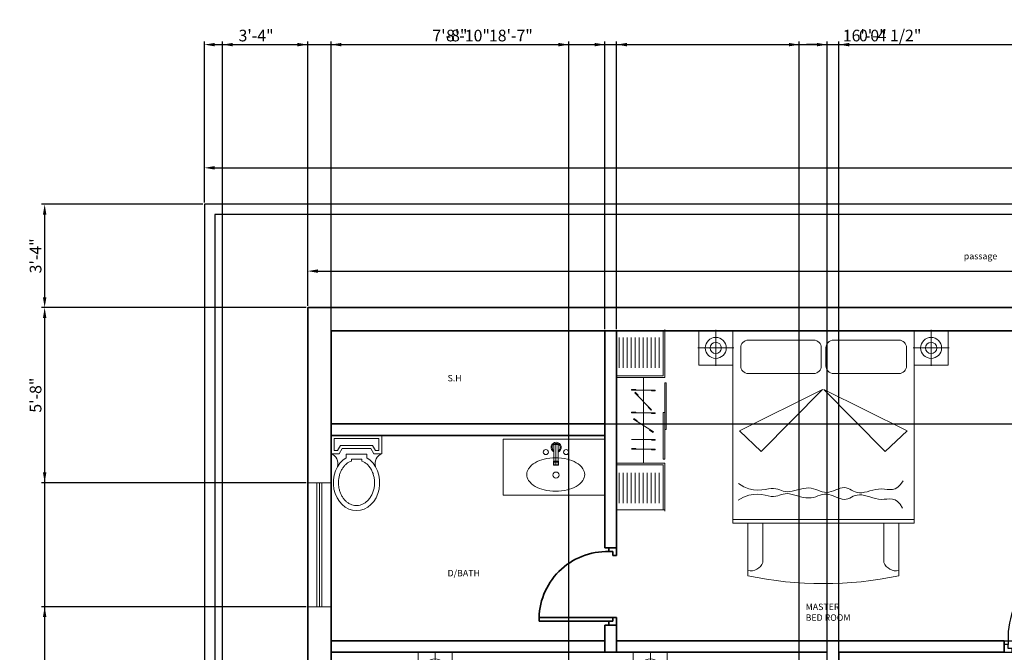
# Model space of a CAD drawing. Units: inches. Extents: x 1239 to 2276906, y 2273 to 321338.
# Tile 17 of 23: x 1239 to 1620, y 3372 to 3617. Entities that reach past the tile are written whole.
import ezdxf

# ---------------------------------------------------------------- set-up
doc = ezdxf.new("R2010")
doc.units = ezdxf.units.IN
for name, color, linetype, lineweight in [('A-ANNO-DIMS', 2, 'Continuous', 18), ('A-AREA-IDEN', 7, 'Continuous', 18), ('A-FLOR-CASE', 8, 'Continuous', 18), ('A-FLOR-FIXT', 9, 'Continuous', 18), ('A-FURN', 8, 'Continuous', 13), ('C-PROP', 7, 'Continuous', 25), ('DOOR', 1, 'Continuous', 25), ('wall', 7, 'Continuous', 35), ('WINDOW', 50, 'Continuous', 18)]:
    doc.layers.add(name, color=color, linetype=linetype, lineweight=lineweight)
doc.styles.get("Standard").update_dxf_attribs({"font": 'arial.ttf'})
doc.dimstyles.new('ISO-25', dxfattribs={"dimtxt": 4.5, "dimasz": 4, "dimexe": 1.25, "dimexo": 0.625, "dimtad": 1, "dimdec": 1, "dimlunit": 3, "dimtxsty": 'Standard', "dimcen": 2.5, "dimadec": 0, "dimazin": 0, "dimtfac": 1, "dimtdec": 1, "dimtmove": 0, "dimatfit": 3, "dimfxl": 1, "dimarcsym": 0})

# ---------------------------------------------------------------- blocks, each defined once
blk = doc.blocks.new('new block')
for p, q in [((1.5, 1.5), (1.5, 30)), ((3, 0), (3, 30)), ((0, 3), (0, 0)), ((1.5, 3), (0, 3)), ((0, 0), (3, 0)), ((1.5, 1.5), (1.5, 3)), ((3, 1.5), (1.5, 1.5)), ((3, 0), (3, 1.5)), ((27, 0), (27, 1.5)), ((27, 1.5), (28.5, 1.5)), ((30, 0), (27, 0)), ((28.5, 1.5), (28.5, 3)), ((28.5, 3), (30, 3)), ((30, 3), (30, 0))]:
    blk.add_line(p, q)
blk.add_arc((2.25, 3.75), 26.26, 358.3634, 91.6366)
blk = doc.blocks.new('2.6door')
at = {"layer": 'wall'}
blk.add_blockref('new block', (0, 0), dxfattribs=at)
blk = doc.blocks.new('A$C7C8779AE')
for p, q in [((0, 0.7405), (0, 0.5605)), ((0.5, 0.7405), (0, 0.7405)), ((0.47, 0.7105), (0.03, 0.7105)), ((0.03, 0.7105), (0.03, 0.5905)), ((0.47, 0.5905), (0.47, 0.7105)), ((0.5, 0.5605), (0.5, 0.7405)), ((0.03, 0.5905), (0.063, 0.5905)), ((0.093, 0.6405), (0.063, 0.5905)), ((0.11, 0.6105), (0.08, 0.5605)), ((0.093, 0.6405), (0.407, 0.6405)), ((0.11, 0.6105), (0.39, 0.6105)), ((0.42, 0.5605), (0.39, 0.6105)), ((0.437, 0.5905), (0.407, 0.6405)), ((0.437, 0.5905), (0.47, 0.5905)), ((0, 0.5605), (0.08, 0.5605)), ((0.1497, 0.557), (0.1497, 0.5203)), ((0.1497, 0.557), (0.3514, 0.557)), ((0.1997, 0.507), (0.1997, 0.4879)), ((0.1997, 0.507), (0.3014, 0.507)), ((0.3014, 0.507), (0.3014, 0.4879)), ((0.3514, 0.557), (0.3514, 0.5203)), ((0.42, 0.5605), (0.5, 0.5605))]:
    blk.add_line(p, q)
for centre, start, end in [((-0.0386, 0.4613), 344.64203, 68.73386), ((0.5386, 0.4613), 111.26614, 195.35797)]:
    blk.add_arc(centre, 0.1064, start, end)
blk.add_ellipse((0.2506, 0.2744), major_axis=(0, 0.2744), ratio=0.828948, start_param=0.459479, end_param=5.823706)
blk.add_open_spline([(0.1997, 0.4879), (0.1697, 0.474), (0.1642, 0.4702), (0.1512, 0.4602), (0.1438, 0.4535), (0.1298, 0.4388), (0.1233, 0.4306), (0.1111, 0.4131), (0.1055, 0.4037), (0.0956, 0.3838), (0.0912, 0.3733), (0.0838, 0.3516), (0.0808, 0.3403), (0.0762, 0.3172), (0.0746, 0.3055), (0.073, 0.2817), (0.0729, 0.2698), (0.0743, 0.246), (0.0758, 0.2342), (0.0801, 0.2111), (0.0831, 0.1998), (0.0903, 0.1779), (0.0945, 0.1673), (0.1043, 0.1473), (0.1098, 0.1378), (0.1218, 0.12), (0.1283, 0.1118), (0.1421, 0.0968), (0.1494, 0.09), (0.1646, 0.078), (0.1725, 0.0728), (0.1887, 0.064), (0.1969, 0.0603), (0.2137, 0.0547), (0.2222, 0.0527), (0.2392, 0.0502), (0.2478, 0.0498), (0.2664, 0.0505), (0.2764, 0.052), (0.2963, 0.0573), (0.3061, 0.061), (0.3253, 0.0707), (0.3346, 0.0766), (0.3525, 0.0906), (0.3611, 0.0987), (0.3771, 0.1169), (0.3845, 0.127), (0.3978, 0.1488), (0.4037, 0.1605), (0.4137, 0.1853), (0.4178, 0.1983), (0.424, 0.2251), (0.4261, 0.2389), (0.4282, 0.2668), (0.4283, 0.2809), (0.4262, 0.3088), (0.4241, 0.3226), (0.418, 0.3495), (0.414, 0.3625), (0.404, 0.3873), (0.3982, 0.3991), (0.385, 0.421), (0.3776, 0.4311), (0.3617, 0.4494), (0.3531, 0.4575), (0.3382, 0.4693), (0.3321, 0.4736), (0.3014, 0.4879)], degree=3, knots=[0.459479, 0.459479, 0.459479, 0.459479, 0.567422, 0.567422, 0.720865, 0.720865, 0.874307, 0.874307, 1.02775, 1.02775, 1.181192, 1.181192, 1.334635, 1.334635, 1.488077, 1.488077, 1.64152, 1.64152, 1.794963, 1.794963, 1.948405, 1.948405, 2.101848, 2.101848, 2.25529, 2.25529, 2.408733, 2.408733, 2.562175, 2.562175, 2.715618, 2.715618, 2.86906, 2.86906, 3.022503, 3.022503, 3.175946, 3.175946, 3.356457, 3.356457, 3.536968, 3.536968, 3.717479, 3.717479, 3.89799, 3.89799, 4.078501, 4.078501, 4.259012, 4.259012, 4.439523, 4.439523, 4.620035, 4.620035, 4.800546, 4.800546, 4.981057, 4.981057, 5.161568, 5.161568, 5.342079, 5.342079, 5.52259, 5.52259, 5.703101, 5.703101, 5.823706, 5.823706, 5.823706, 5.823706])
blk = doc.blocks.new('A$C50A015BB')
for p, q in [((0, 0.55), (1, 0.55)), ((0, 0.55), (0, 0)), ((0.4985, 0.5), (0.5385, 0.5)), ((0.4985, 0.5), (0.4985, 0.3)), ((0.5185, 0.5), (0.5185, 0.3)), ((0.5385, 0.5), (0.5385, 0.3)), ((1, 0.55), (1, 0)), ((0.4935, 0.335), (0.4935, 0.295)), ((0.4935, 0.335), (0.5435, 0.335)), ((0.4935, 0.295), (0.5435, 0.295)), ((0.4985, 0.325), (0.5385, 0.325)), ((0.4985, 0.3), (0.5385, 0.3)), ((0.5435, 0.335), (0.5435, 0.295)), ((0, 0), (1, 0)), ((0, 0), (1, 0))]:
    blk.add_line(p, q)
for centre, radius in [((0.4185, 0.424), 0.025), ((0.6185, 0.424), 0.025), ((0.5185, 0.1981), 0.0298)]:
    blk.add_circle(centre, radius)
for centre, radius, start, end in [((0.5201, 0.4703), 0.0497, 291.74253, 244.23308), ((0.5201, 0.4703), 0.0397, 297.63203, 237.02558), ((0.4185, 0.1397), 0.2081, 120.06859, 144.41781), ((0.4772, 0.0383), 0.3252, 103.48533, 120.06859), ((0.5157, -0.1225), 0.4906, 90, 103.48533), ((0.5157, -0.1225), 0.4906, 76.51467, 90), ((0.5543, 0.0383), 0.3252, 59.93141, 76.51467), ((0.613, 0.1397), 0.2081, 35.58219, 59.93141), ((0.3299, 0.2031), 0.0991, 144.41781, 180), ((0.3299, 0.2031), 0.0991, 180, 215.58219), ((0.7016, 0.2031), 0.0991, 0, 35.58219), ((0.7016, 0.2031), 0.0991, 324.41781, 0), ((0.4185, 0.2665), 0.2081, 215.58219, 239.93141), ((0.613, 0.2665), 0.2081, 300.06859, 324.41781), ((0.4772, 0.3679), 0.3252, 239.93141, 256.51467), ((0.5157, 0.5288), 0.4906, 256.51467, 270), ((0.5157, 0.5288), 0.4906, 270, 283.48533), ((0.5543, 0.3679), 0.3252, 283.48533, 300.06859)]:
    blk.add_arc(centre, radius, start, end)
blk = doc.blocks.new('A$C4F543DC7')
for p, q in [((0.013, 3.35, -0.169), (3.313, 3.35, -0.169)), ((0.463, 3.35, -0.169), (0.013, 3.35, -0.169)), ((0.013, 2.896, -0.169), (0.013, 3.35, -0.169)), ((0.013, 3.35, -0.169), (0.013, 2.896, -0.169)), ((0.238, 3.123, -0.439), (0.238, 3.361, -0.439)), ((0.463, 3.35, -0.169), (0.463, 0.8, -0.169)), ((2.863, 3.35, -0.169), (0.463, 3.35, -0.169)), ((0.463, 2.896, -0.169), (0.463, 3.35, -0.169)), ((2.863, 0.8, -0.169), (2.863, 3.35, -0.169)), ((2.863, 3.35, -0.169), (3.313, 3.35, -0.169)), ((2.863, 2.896, -0.169), (2.863, 3.35, -0.169)), ((3.089, 3.123, -0.439), (3.089, 3.361, -0.439)), ((3.313, 3.35, -0.169), (3.313, 2.896, -0.169)), ((3.313, 3.35, -0.169), (3.313, 2.896, -0.169)), ((1.535, 3.226, -0.169), (0.668, 3.226, -0.169)), ((2.664, 3.226, -0.169), (1.797, 3.226, -0.169)), ((0.238, 3.123, -0.439), (0, 3.123, -0.439)), ((0.238, 3.123, -0.439), (0.476, 3.123, -0.439)), ((0.238, 3.123, -0.439), (0.238, 2.885, -0.439)), ((0.568, 3.126, -0.169), (0.568, 2.884, -0.169)), ((1.635, 2.884, -0.169), (1.635, 3.126, -0.169)), ((1.697, 3.126, -0.169), (1.697, 2.884, -0.169)), ((2.764, 2.884, -0.169), (2.764, 3.126, -0.169)), ((3.089, 3.123, -0.439), (2.851, 3.123, -0.439)), ((3.089, 3.123, -0.439), (3.089, 2.885, -0.439)), ((3.089, 3.123, -0.439), (3.327, 3.123, -0.439)), ((0.463, 2.896, -0.169), (0.013, 2.896, -0.169)), ((0.013, 2.896, -0.169), (0.463, 2.896, -0.169)), ((0.463, 0.8, -0.169), (0.463, 2.896, -0.169)), ((2.863, 2.896, -0.169), (2.863, 0.8, -0.169)), ((3.313, 2.896, -0.169), (2.863, 2.896, -0.169)), ((3.313, 2.896, -0.169), (2.863, 2.896, -0.169)), ((0.668, 2.784, -0.169), (1.535, 2.784, -0.169)), ((1.797, 2.784, -0.169), (2.664, 2.784, -0.169)), ((1.653, 2.573, -0.169), (0.55, 2.025, -0.169)), ((0.841, 1.752, -0.169), (1.653, 2.573, -0.169)), ((2.481, 1.752, -0.169), (1.669, 2.573, -0.169)), ((1.669, 2.573, -0.169), (2.772, 2.025, -0.169)), ((0.55, 2.025, -0.169), (0.841, 1.752, -0.169)), ((2.772, 2.025, -0.169), (2.481, 1.752, -0.169)), ((0.537, 1.327, -0.169), (0.609, 1.284, -0.169)), ((2.648, 1.277, -0.169), (2.683, 1.312, -0.169)), ((2.683, 1.312, -0.169), (2.718, 1.364, -0.169)), ((0.609, 1.284, -0.169), (0.676, 1.257, -0.169)), ((0.674, 1.171, -0.169), (0.736, 1.183, -0.169)), ((0.676, 1.257, -0.169), (0.737, 1.243, -0.169)), ((0.736, 1.183, -0.169), (0.793, 1.185, -0.169)), ((0.737, 1.243, -0.169), (0.794, 1.239, -0.169)), ((0.793, 1.185, -0.169), (0.845, 1.18, -0.169)), ((0.794, 1.239, -0.169), (0.846, 1.242, -0.169)), ((0.845, 1.18, -0.169), (0.891, 1.172, -0.169)), ((0.846, 1.242, -0.169), (0.893, 1.249, -0.169)), ((0.893, 1.249, -0.169), (0.935, 1.256, -0.169)), ((0.935, 1.256, -0.169), (0.972, 1.261, -0.169)), ((0.972, 1.261, -0.169), (1.004, 1.262, -0.169)), ((1.004, 1.262, -0.169), (1.033, 1.258, -0.169)), ((1.033, 1.258, -0.169), (1.06, 1.251, -0.169)), ((1.06, 1.251, -0.169), (1.084, 1.242, -0.169)), ((1.083, 1.172, -0.169), (1.107, 1.18, -0.169)), ((1.084, 1.242, -0.169), (1.108, 1.234, -0.169)), ((1.107, 1.18, -0.169), (1.132, 1.187, -0.169)), ((1.108, 1.234, -0.169), (1.132, 1.226, -0.169)), ((1.132, 1.226, -0.169), (1.158, 1.22, -0.169)), ((1.132, 1.187, -0.169), (1.157, 1.192, -0.169)), ((1.157, 1.192, -0.169), (1.185, 1.193, -0.169)), ((1.158, 1.22, -0.169), (1.185, 1.218, -0.169)), ((1.185, 1.218, -0.169), (1.216, 1.22, -0.169)), ((1.185, 1.193, -0.169), (1.216, 1.19, -0.169)), ((1.216, 1.22, -0.169), (1.25, 1.226, -0.169)), ((1.216, 1.19, -0.169), (1.249, 1.183, -0.169)), ((1.249, 1.183, -0.169), (1.284, 1.173, -0.169)), ((1.25, 1.226, -0.169), (1.285, 1.235, -0.169)), ((1.284, 1.173, -0.169), (1.321, 1.163, -0.169)), ((1.285, 1.235, -0.169), (1.322, 1.244, -0.169)), ((1.322, 1.244, -0.169), (1.359, 1.253, -0.169)), ((1.359, 1.253, -0.169), (1.396, 1.261, -0.169)), ((1.396, 1.261, -0.169), (1.433, 1.266, -0.169)), ((1.433, 1.266, -0.169), (1.468, 1.268, -0.169)), ((1.468, 1.268, -0.169), (1.501, 1.264, -0.169)), ((1.501, 1.264, -0.169), (1.532, 1.257, -0.169)), ((1.532, 1.257, -0.169), (1.562, 1.247, -0.169)), ((1.562, 1.247, -0.169), (1.591, 1.237, -0.169)), ((1.591, 1.237, -0.169), (1.62, 1.226, -0.169)), ((1.619, 1.172, -0.169), (1.648, 1.18, -0.169)), ((1.62, 1.226, -0.169), (1.648, 1.217, -0.169)), ((1.648, 1.217, -0.169), (1.676, 1.211, -0.169)), ((1.648, 1.18, -0.169), (1.676, 1.185, -0.169)), ((1.676, 1.211, -0.169), (1.705, 1.209, -0.169)), ((1.676, 1.185, -0.169), (1.705, 1.186, -0.169)), ((1.705, 1.209, -0.169), (1.735, 1.212, -0.169)), ((1.705, 1.186, -0.169), (1.734, 1.182, -0.169)), ((1.734, 1.182, -0.169), (1.764, 1.173, -0.169)), ((1.735, 1.212, -0.169), (1.765, 1.22, -0.169)), ((1.765, 1.22, -0.169), (1.795, 1.23, -0.169)), ((1.795, 1.23, -0.169), (1.826, 1.242, -0.169)), ((1.826, 1.242, -0.169), (1.856, 1.253, -0.169)), ((1.856, 1.253, -0.169), (1.885, 1.263, -0.169)), ((1.885, 1.263, -0.169), (1.913, 1.27, -0.169)), ((1.913, 1.27, -0.169), (1.94, 1.272, -0.169)), ((1.94, 1.272, -0.169), (1.965, 1.269, -0.169)), ((1.965, 1.269, -0.169), (1.989, 1.262, -0.169)), ((1.989, 1.262, -0.169), (2.012, 1.251, -0.169)), ((2.012, 1.251, -0.169), (2.036, 1.239, -0.169)), ((2.036, 1.239, -0.169), (2.06, 1.227, -0.169)), ((2.06, 1.227, -0.169), (2.085, 1.216, -0.169)), ((2.084, 1.167, -0.169), (2.111, 1.174, -0.169)), ((2.085, 1.216, -0.169), (2.112, 1.208, -0.169)), ((2.111, 1.174, -0.169), (2.14, 1.177, -0.169)), ((2.112, 1.208, -0.169), (2.141, 1.204, -0.169)), ((2.14, 1.177, -0.169), (2.172, 1.175, -0.169)), ((2.141, 1.204, -0.169), (2.172, 1.205, -0.169)), ((2.172, 1.205, -0.169), (2.206, 1.21, -0.169)), ((2.172, 1.175, -0.169), (2.206, 1.169, -0.169)), ((2.206, 1.21, -0.169), (2.242, 1.218, -0.169)), ((2.242, 1.218, -0.169), (2.279, 1.228, -0.169)), ((2.279, 1.228, -0.169), (2.317, 1.238, -0.169)), ((2.317, 1.238, -0.169), (2.356, 1.246, -0.169)), ((2.356, 1.246, -0.169), (2.394, 1.253, -0.169)), ((2.394, 1.253, -0.169), (2.433, 1.255, -0.169)), ((2.433, 1.255, -0.169), (2.47, 1.253, -0.169)), ((2.47, 1.253, -0.169), (2.506, 1.249, -0.169)), ((2.506, 1.249, -0.169), (2.542, 1.246, -0.169)), ((2.542, 1.246, -0.169), (2.578, 1.248, -0.169)), ((2.578, 1.248, -0.169), (2.613, 1.257, -0.169)), ((2.613, 1.257, -0.169), (2.648, 1.277, -0.169)), ((0.533, 1.105, -0.169), (0.607, 1.146, -0.169)), ((0.607, 1.146, -0.169), (0.674, 1.171, -0.169)), ((0.891, 1.172, -0.169), (0.933, 1.163, -0.169)), ((0.933, 1.163, -0.169), (0.97, 1.156, -0.169)), ((0.97, 1.156, -0.169), (1.003, 1.155, -0.169)), ((1.003, 1.155, -0.169), (1.032, 1.158, -0.169)), ((1.032, 1.158, -0.169), (1.058, 1.164, -0.169)), ((1.058, 1.164, -0.169), (1.083, 1.172, -0.169)), ((1.321, 1.163, -0.169), (1.358, 1.152, -0.169)), ((1.358, 1.152, -0.169), (1.394, 1.143, -0.169)), ((1.394, 1.143, -0.169), (1.431, 1.137, -0.169)), ((1.431, 1.137, -0.169), (1.466, 1.135, -0.169)), ((1.466, 1.135, -0.169), (1.499, 1.137, -0.169)), ((1.499, 1.137, -0.169), (1.531, 1.143, -0.169)), ((1.531, 1.143, -0.169), (1.561, 1.152, -0.169)), ((1.561, 1.152, -0.169), (1.59, 1.162, -0.169)), ((1.59, 1.162, -0.169), (1.619, 1.172, -0.169)), ((1.764, 1.173, -0.169), (1.794, 1.162, -0.169)), ((1.794, 1.162, -0.169), (1.824, 1.149, -0.169)), ((1.824, 1.149, -0.169), (1.854, 1.137, -0.169)), ((1.854, 1.137, -0.169), (1.883, 1.126, -0.169)), ((1.883, 1.126, -0.169), (1.911, 1.119, -0.169)), ((1.911, 1.119, -0.169), (1.937, 1.115, -0.169)), ((1.937, 1.115, -0.169), (1.963, 1.118, -0.169)), ((1.963, 1.118, -0.169), (1.987, 1.124, -0.169)), ((1.987, 1.124, -0.169), (2.011, 1.134, -0.169)), ((2.011, 1.134, -0.169), (2.034, 1.145, -0.169)), ((2.034, 1.145, -0.169), (2.059, 1.157, -0.169)), ((2.059, 1.157, -0.169), (2.084, 1.167, -0.169)), ((2.206, 1.169, -0.169), (2.241, 1.16, -0.169)), ((2.241, 1.16, -0.169), (2.278, 1.149, -0.169)), ((2.278, 1.149, -0.169), (2.316, 1.138, -0.169)), ((2.316, 1.138, -0.169), (2.354, 1.128, -0.169)), ((2.354, 1.128, -0.169), (2.392, 1.121, -0.169)), ((2.392, 1.121, -0.169), (2.43, 1.117, -0.169)), ((2.43, 1.117, -0.169), (2.468, 1.118, -0.169)), ((2.468, 1.118, -0.169), (2.504, 1.121, -0.169)), ((2.504, 1.121, -0.169), (2.54, 1.123, -0.169)), ((2.54, 1.123, -0.169), (2.576, 1.12, -0.169)), ((2.576, 1.12, -0.169), (2.611, 1.109, -0.169)), ((2.611, 1.109, -0.169), (2.645, 1.088, -0.169)), ((2.645, 1.088, -0.169), (2.679, 1.052, -0.169)), ((2.679, 1.052, -0.169), (2.712, 0.999, -0.169)), ((0.463, 0.85, -0.169), (2.863, 0.85, -0.169)), ((0.463, 0.8, -0.169), (2.863, 0.8, -0.169)), ((0.663, 0.8, -0.169), (0.463, 0.8, -0.169)), ((0.663, 0.8, -0.169), (2.663, 0.8, -0.169)), ((0.663, 0.104, -0.169), (0.663, 0.8, -0.169)), ((0.663, 0.104, -0.169), (0.663, 0.8, -0.169)), ((0.863, 0.281, -0.169), (0.863, 0.8, -0.169)), ((2.463, 0.8, -0.169), (2.463, 0.281, -0.169)), ((2.863, 0.8, -0.169), (2.663, 0.8, -0.169)), ((2.663, 0.8, -0.169), (2.663, 0.104, -0.169)), ((2.663, 0.8, -0.169), (2.663, 0.104, -0.169))]:
    blk.add_line(p, q)
for centre, radius in [((0.238, 3.123, -0.439), 0.139), ((3.089, 3.123, -0.439), 0.139), ((0.238, 3.123, -0.439), 0.075), ((3.089, 3.123, -0.439), 0.075)]:
    blk.add_circle(centre, radius)
for centre, radius, start, end in [((0.668, 3.126, -0.169), 0.1, 90, 180), ((1.535, 3.126, -0.169), 0.1, 0, 90), ((1.797, 3.126, -0.169), 0.1, 90, 180), ((2.664, 3.126, -0.169), 0.1, 0, 90), ((0.668, 2.884, -0.169), 0.1, 180, 270), ((1.535, 2.884, -0.169), 0.1, 270, 0), ((1.797, 2.884, -0.169), 0.1, 180, 270), ((2.664, 2.884, -0.169), 0.1, 270, 0), ((0.699, 0.347, -0.169), 0.177, 258.2616, 338.032), ((2.627, 0.347, -0.169), 0.177, 201.968, 281.7384), ((1.663, 4.86, -0.169), 4.86, 258.1252, 281.8748), ((1.663, 4.86, -0.169), 4.86, 258.1252, 281.8748)]:
    blk.add_arc(centre, radius, start, end)
blk = doc.blocks.new('A$C34930FF8')
at = {"ltscale": 0.05}
for p, q in [((0, 2252), (0, 17)), ((600, 2252), (0, 2252)), ((185, 1513), (185, 1521)), ((227, 1479), (233, 1485)), ((238, 1513), (238, 1521)), ((437, 1513), (437, 1504)), ((482, 1513), (482, 1504)), ((264, 1442), (270, 1448)), ((185, 1229), (185, 1238)), ((238, 1229), (238, 1238)), ((398, 1304), (392, 1298)), ((435, 1266), (429, 1260)), ((209, 1150), (214, 1157)), ((253, 1122), (258, 1129)), ((437, 1228), (437, 1220)), ((482, 1228), (482, 1220)), ((415, 1018), (411, 1010)), ((459, 989), (455, 982)), ((482, 895), (482, 886)), ((238, 775), (238, 784)), ((437, 775), (437, 767)), ((482, 775), (482, 767)), ((600, 17), (0, 17))]:
    blk.add_line(p, q, dxfattribs=at)
for p, q in [((580, 1691), (580, 2252)), ((600, 1669), (600, 2269)), ((30, 1791), (30, 2169)), ((80, 1791), (80, 2169)), ((130, 1791), (130, 2169)), ((180, 1791), (180, 2169)), ((230, 1791), (230, 2169)), ((280, 1791), (280, 2169)), ((330, 1791), (330, 2169)), ((380, 1791), (380, 2169)), ((430, 1791), (430, 2169)), ((480, 1791), (480, 2169)), ((530, 1791), (530, 2169)), ((580, 1691), (0, 1691)), ((600, 1669), (0, 1669)), ((335, 1666), (335, 603)), ((600, 1603), (620, 1603)), ((600, 1019), (600, 1603)), ((620, 1603), (620, 1019)), ((238, 1521), (185, 1521)), ((482, 1513), (185, 1513)), ((435, 1266), (227, 1479)), ((270, 1448), (233, 1485)), ((437, 1504), (482, 1504)), ((238, 1238), (185, 1238)), ((429, 1260), (392, 1298)), ((600, 1233), (580, 1233)), ((580, 1233), (580, 649)), ((600, 649), (600, 1233)), ((482, 1228), (185, 1228)), ((459, 989), (209, 1150)), ((258, 1129), (214, 1157)), ((437, 1220), (482, 1220)), ((455, 982), (411, 1010)), ((620, 1019), (600, 1019)), ((482, 895), (185, 895)), ((437, 886), (482, 886)), ((238, 784), (185, 784)), ((482, 775), (185, 775)), ((437, 767), (482, 767)), ((580, 649), (600, 649)), ((600, 600), (0, 600)), ((580, 578), (0, 578)), ((580, 578), (580, 17)), ((600, 600), (600, 0)), ((30, 478), (30, 100)), ((80, 478), (80, 100)), ((130, 478), (130, 100)), ((180, 478), (180, 100)), ((230, 478), (230, 100)), ((280, 478), (280, 100)), ((330, 478), (330, 100)), ((380, 478), (380, 100)), ((430, 478), (430, 100)), ((480, 478), (480, 100)), ((530, 478), (530, 100))]:
    blk.add_line(p, q)
blk = doc.blocks.new('*D37')
at = {"layer": 'A-ANNO-DIMS', "color": 0, "lineweight": -2, "transparency": 16777216}
for p, q in [((1310.38, 3546.52), (1310.38, 3561.25)), ((1314.38, 3560), (1966.38, 3560)), ((1970.38, 3546.52), (1970.38, 3561.25))]:
    blk.add_line(p, q, dxfattribs=at)
at = {"layer": 'A-ANNO-DIMS', "color": 0, "transparency": 16777216}
for points in [[(1314.38, 3560.67), (1314.38, 3559.33), (1310.38, 3560)], [(1966.38, 3560.67), (1966.38, 3559.33), (1970.38, 3560)]]:
    blk.add_solid(points, dxfattribs=at)
at = {"layer": 'Defpoints', "color": 0, "transparency": 16777216}
for p in [(1970.38, 3560), (1310.38, 3545.9), (1970.38, 3545.9)]:
    blk.add_point(p, dxfattribs=at)
at = {"layer": 'A-ANNO-DIMS', "color": 0, "transparency": 16777216, "insert": (1640.38, 3562.91), "char_height": 4.5, "attachment_point": 5}
blk.add_mtext("55'", dxfattribs=at)
blk = doc.blocks.new('*D39')
at = {"layer": 'A-ANNO-DIMS', "color": 0, "lineweight": -2, "transparency": 16777216}
for p, q in [((1350.38, 3506.52), (1350.38, 3521.25)), ((1930.38, 3506.52), (1930.38, 3521.25)), ((1354.38, 3520), (1926.38, 3520))]:
    blk.add_line(p, q, dxfattribs=at)
at = {"layer": 'A-ANNO-DIMS', "color": 0, "transparency": 16777216}
for points in [[(1354.38, 3520.67), (1354.38, 3519.33), (1350.38, 3520)], [(1926.38, 3520.67), (1926.38, 3519.33), (1930.38, 3520)]]:
    blk.add_solid(points, dxfattribs=at)
at = {"layer": 'Defpoints', "color": 0, "transparency": 16777216}
for p in [(1930.38, 3520), (1350.38, 3505.9), (1930.38, 3505.9)]:
    blk.add_point(p, dxfattribs=at)
at = {"layer": 'A-ANNO-DIMS', "color": 0, "transparency": 16777216, "insert": (1640.38, 3522.92), "char_height": 4.5, "attachment_point": 5}
blk.add_mtext('48\'-4"', dxfattribs=at)
blk = doc.blocks.new('DOOR-SINGLE-36')
for p, q in [((33, 1.5), (33, 37.5)), ((34.5, 1.5), (34.5, 37.5)), ((0, 3), (0, 0)), ((1.5, 3), (0, 3)), ((0, 0), (3, 0)), ((1.5, 1.5), (1.5, 3)), ((3, 1.5), (1.5, 1.5)), ((3, 0), (3, 1.5)), ((33, 0), (33, 1.5)), ((33, 1.5), (34.5, 1.5)), ((36, 0), (33, 0)), ((34.5, 1.5), (34.5, 3)), ((34.5, 3), (36, 3)), ((36, 3), (36, 0))]:
    blk.add_line(p, q)
blk.add_arc((33.75, 5.18), 32.32, 88.6705, 183.8756)
blk = doc.blocks.new('WIN-48')
for p, q in [((0, 48), (9, 48)), ((0, 0), (0, 48)), ((3.5, 0), (3.5, 48)), ((4.5, 0), (4.5, 48)), ((5.5, 0), (5.5, 48)), ((9, 0), (9, 48)), ((0, 0), (9, 0))]:
    blk.add_line(p, q)
blk = doc.blocks.new('*D80')
at = {"layer": 'A-ANNO-DIMS', "color": 0, "lineweight": -2, "transparency": 16777216}
for p, q in [((1310.38, 3546.52), (1310.38, 3608.95)), ((1350.38, 3506.52), (1350.38, 3608.95)), ((1314.38, 3607.7), (1346.38, 3607.7))]:
    blk.add_line(p, q, dxfattribs=at)
at = {"layer": 'A-ANNO-DIMS', "color": 0, "transparency": 16777216}
for points in [[(1314.38, 3608.36), (1314.38, 3607.03), (1310.38, 3607.7)], [(1346.38, 3608.36), (1346.38, 3607.03), (1350.38, 3607.7)]]:
    blk.add_solid(points, dxfattribs=at)
at = {"layer": 'Defpoints', "color": 0, "transparency": 16777216}
for p in [(1350.38, 3607.7), (1310.38, 3545.9), (1350.38, 3505.9)]:
    blk.add_point(p, dxfattribs=at)
at = {"layer": 'A-ANNO-DIMS', "color": 0, "transparency": 16777216, "insert": (1330.38, 3610.62), "char_height": 4.5, "attachment_point": 5}
blk.add_mtext('3\'-4"', dxfattribs=at)
blk = doc.blocks.new('*D81')
at = {"layer": 'A-ANNO-DIMS', "color": 0, "lineweight": -2, "transparency": 16777216}
for p, q in [((1309.76, 3545.9), (1247.33, 3545.9)), ((1248.58, 3541.9), (1248.58, 3509.9)), ((1349.76, 3505.9), (1247.33, 3505.9))]:
    blk.add_line(p, q, dxfattribs=at)
at = {"layer": 'A-ANNO-DIMS', "color": 0, "transparency": 16777216}
for points in [[(1247.92, 3541.9), (1249.25, 3541.9), (1248.58, 3545.9)], [(1247.92, 3509.9), (1249.25, 3509.9), (1248.58, 3505.9)]]:
    blk.add_solid(points, dxfattribs=at)
at = {"layer": 'Defpoints', "color": 0, "transparency": 16777216}
for p in [(1310.38, 3545.9), (1248.58, 3505.9), (1350.38, 3505.9)]:
    blk.add_point(p, dxfattribs=at)
at = {"layer": 'A-ANNO-DIMS', "color": 0, "transparency": 16777216, "insert": (1245.66, 3525.9), "char_height": 4.5, "attachment_point": 5, "rotation": 90}
blk.add_mtext('3\'-4"', dxfattribs=at)
blk = doc.blocks.new('*D82')
at = {"layer": 'A-ANNO-DIMS', "color": 0, "lineweight": -2, "transparency": 16777216}
for p, q in [((1349.76, 3505.9), (1247.33, 3505.9)), ((1248.58, 3501.9), (1248.58, 2634.4)), ((1358.76, 2630.4), (1247.33, 2630.4))]:
    blk.add_line(p, q, dxfattribs=at)
at = {"layer": 'A-ANNO-DIMS', "color": 0, "transparency": 16777216}
for points in [[(1247.92, 3501.9), (1249.25, 3501.9), (1248.58, 3505.9)], [(1247.92, 2634.4), (1249.25, 2634.4), (1248.58, 2630.4)]]:
    blk.add_solid(points, dxfattribs=at)
at = {"layer": 'Defpoints', "color": 0, "transparency": 16777216}
for p in [(1350.38, 3505.9), (1248.58, 2630.4), (1359.38, 2630.4)]:
    blk.add_point(p, dxfattribs=at)
at = {"layer": 'A-ANNO-DIMS', "color": 0, "transparency": 16777216, "insert": (1245.63, 3068.15), "char_height": 4.5, "attachment_point": 5, "rotation": 90}
blk.add_mtext('72\'-11 1/2"', dxfattribs=at)
blk = doc.blocks.new('*D83')
at = {"layer": 'A-ANNO-DIMS', "color": 0, "lineweight": -2, "transparency": 16777216}
for p, q in [((1359.38, 3497.52), (1359.38, 3608.95)), ((1465.38, 3497.52), (1465.38, 3608.95)), ((1363.38, 3607.7), (1461.38, 3607.7))]:
    blk.add_line(p, q, dxfattribs=at)
at = {"layer": 'A-ANNO-DIMS', "color": 0, "transparency": 16777216}
for points in [[(1363.38, 3608.36), (1363.38, 3607.03), (1359.38, 3607.7)], [(1461.38, 3608.36), (1461.38, 3607.03), (1465.38, 3607.7)]]:
    blk.add_solid(points, dxfattribs=at)
at = {"layer": 'Defpoints', "color": 0, "transparency": 16777216}
for p in [(1465.38, 3607.7), (1359.38, 3496.9), (1465.38, 3496.9)]:
    blk.add_point(p, dxfattribs=at)
at = {"layer": 'A-ANNO-DIMS', "color": 0, "transparency": 16777216, "insert": (1412.38, 3610.62), "char_height": 4.5, "attachment_point": 5}
blk.add_mtext('8\'-10"', dxfattribs=at)
blk = doc.blocks.new('*D84')
at = {"layer": 'A-ANNO-DIMS', "color": 0, "lineweight": -2, "transparency": 16777216}
for p, q in [((1469.88, 3497.52), (1469.88, 3608.95)), ((1661.88, 3497.52), (1661.88, 3608.95)), ((1473.88, 3607.7), (1657.88, 3607.7))]:
    blk.add_line(p, q, dxfattribs=at)
at = {"layer": 'A-ANNO-DIMS', "color": 0, "transparency": 16777216}
for points in [[(1473.88, 3608.36), (1473.88, 3607.03), (1469.88, 3607.7)], [(1657.88, 3608.36), (1657.88, 3607.03), (1661.88, 3607.7)]]:
    blk.add_solid(points, dxfattribs=at)
at = {"layer": 'Defpoints', "color": 0, "transparency": 16777216}
for p in [(1661.88, 3607.7), (1469.88, 3496.9), (1661.88, 3496.9)]:
    blk.add_point(p, dxfattribs=at)
at = {"layer": 'A-ANNO-DIMS', "color": 0, "transparency": 16777216, "insert": (1565.88, 3610.62), "char_height": 4.5, "attachment_point": 5}
blk.add_mtext('16\'-0"', dxfattribs=at)
blk = doc.blocks.new('*D85')
at = {"layer": 'A-ANNO-DIMS', "color": 0, "lineweight": -2, "transparency": 16777216}
for p, q in [((1470.51, 3496.9), (2033.43, 3496.9)), ((2032.18, 3380.9), (2032.18, 3492.9)), ((1470.51, 3376.9), (2033.43, 3376.9))]:
    blk.add_line(p, q, dxfattribs=at)
at = {"layer": 'A-ANNO-DIMS', "color": 0, "transparency": 16777216}
for points in [[(2031.52, 3492.9), (2032.85, 3492.9), (2032.18, 3496.9)], [(2031.52, 3380.9), (2032.85, 3380.9), (2032.18, 3376.9)]]:
    blk.add_solid(points, dxfattribs=at)
at = {"layer": 'Defpoints', "color": 0, "transparency": 16777216}
for p in [(1469.88, 3496.9), (2032.18, 3496.9), (1469.88, 3376.9)]:
    blk.add_point(p, dxfattribs=at)
at = {"layer": 'A-ANNO-DIMS', "color": 0, "transparency": 16777216, "insert": (2029.26, 3436.9), "char_height": 4.5, "attachment_point": 5, "rotation": 90}
blk.add_mtext('10\'-0"', dxfattribs=at)
blk = doc.blocks.new('*D91')
at = {"layer": 'A-ANNO-DIMS', "color": 0, "lineweight": -2, "transparency": 16777216}
for p, q in [((1359.38, 3116.52), (1359.38, 3608.95)), ((1451.38, 3106.02), (1451.38, 3608.95)), ((1363.38, 3607.7), (1447.38, 3607.7))]:
    blk.add_line(p, q, dxfattribs=at)
at = {"layer": 'A-ANNO-DIMS', "color": 0, "transparency": 16777216}
for points in [[(1363.38, 3608.36), (1363.38, 3607.03), (1359.38, 3607.7)], [(1447.38, 3608.36), (1447.38, 3607.03), (1451.38, 3607.7)]]:
    blk.add_solid(points, dxfattribs=at)
at = {"layer": 'Defpoints', "color": 0, "transparency": 16777216}
for p in [(1451.38, 3607.7), (1359.38, 3115.9), (1451.38, 3105.4)]:
    blk.add_point(p, dxfattribs=at)
at = {"layer": 'A-ANNO-DIMS', "color": 0, "transparency": 16777216, "insert": (1405.38, 3610.62), "char_height": 4.5, "attachment_point": 5}
blk.add_mtext('7\'-8"', dxfattribs=at)
blk = doc.blocks.new('*D102')
at = {"layer": 'A-ANNO-DIMS', "color": 0, "lineweight": -2, "transparency": 16777216}
for p, q in [((1317.38, 2608.14), (1317.38, 3608.95)), ((1540.55, 2608.14), (1540.55, 3608.95)), ((1321.38, 3607.7), (1536.55, 3607.7))]:
    blk.add_line(p, q, dxfattribs=at)
at = {"layer": 'A-ANNO-DIMS', "color": 0, "transparency": 16777216}
for points in [[(1321.38, 3608.36), (1321.38, 3607.03), (1317.38, 3607.7)], [(1536.55, 3608.36), (1536.55, 3607.03), (1540.55, 3607.7)]]:
    blk.add_solid(points, dxfattribs=at)
at = {"layer": 'Defpoints', "color": 0, "transparency": 16777216}
for p in [(1540.55, 3607.7), (1317.38, 2607.52), (1540.55, 2607.52)]:
    blk.add_point(p, dxfattribs=at)
at = {"layer": 'A-ANNO-DIMS', "color": 0, "transparency": 16777216, "insert": (1428.97, 3610.62), "char_height": 4.5, "attachment_point": 5}
blk.add_mtext('18\'-7"', dxfattribs=at)
blk = doc.blocks.new('*D104')
at = {"layer": 'A-ANNO-DIMS', "color": 0, "lineweight": -2, "transparency": 16777216}
for p, q in [((1349.76, 3505.9), (1247.33, 3505.9)), ((1248.58, 3501.9), (1248.58, 3442.05)), ((1349.76, 3438.05), (1247.33, 3438.05))]:
    blk.add_line(p, q, dxfattribs=at)
at = {"layer": 'A-ANNO-DIMS', "color": 0, "transparency": 16777216}
for points in [[(1247.92, 3501.9), (1249.25, 3501.9), (1248.58, 3505.9)], [(1247.92, 3442.05), (1249.25, 3442.05), (1248.58, 3438.05)]]:
    blk.add_solid(points, dxfattribs=at)
at = {"layer": 'Defpoints', "color": 0, "transparency": 16777216}
for p in [(1350.38, 3505.9), (1248.58, 3438.05), (1350.38, 3438.05)]:
    blk.add_point(p, dxfattribs=at)
at = {"layer": 'A-ANNO-DIMS', "color": 0, "transparency": 16777216, "insert": (1245.66, 3471.97), "char_height": 4.5, "attachment_point": 5, "rotation": 90}
blk.add_mtext('5\'-8"', dxfattribs=at)
blk = doc.blocks.new('*D105')
at = {"layer": 'A-ANNO-DIMS', "color": 0, "lineweight": -2, "transparency": 16777216}
for p, q in [((1349.76, 3390.05), (1247.33, 3390.05)), ((1248.58, 3386.05), (1248.58, 3313.78)), ((1349.76, 3309.78), (1247.33, 3309.78))]:
    blk.add_line(p, q, dxfattribs=at)
at = {"layer": 'A-ANNO-DIMS', "color": 0, "transparency": 16777216}
for points in [[(1247.92, 3386.05), (1249.25, 3386.05), (1248.58, 3390.05)], [(1247.92, 3313.78), (1249.25, 3313.78), (1248.58, 3309.78)]]:
    blk.add_solid(points, dxfattribs=at)
at = {"layer": 'Defpoints', "color": 0, "transparency": 16777216}
for p in [(1350.38, 3390.05), (1248.58, 3309.78), (1350.38, 3309.78)]:
    blk.add_point(p, dxfattribs=at)
at = {"layer": 'A-ANNO-DIMS', "color": 0, "transparency": 16777216, "insert": (1245.63, 3349.91), "char_height": 4.5, "attachment_point": 5, "rotation": 90}
blk.add_mtext('6\'-8 1/2"', dxfattribs=at)
blk = doc.blocks.new('*D111')
at = {"layer": 'A-ANNO-DIMS', "color": 0, "lineweight": -2, "transparency": 16777216}
for p, q in [((1551.38, 2635.52), (1551.38, 3608.95)), ((1555.88, 2631.02), (1555.88, 3608.95)), ((1547.38, 3607.7), (1543.38, 3607.7)), ((1551.38, 3607.7), (1555.88, 3607.7)), ((1559.88, 3607.7), (1587.58, 3607.7))]:
    blk.add_line(p, q, dxfattribs=at)
at = {"layer": 'A-ANNO-DIMS', "color": 0, "transparency": 16777216}
for points in [[(1547.38, 3608.36), (1547.38, 3607.03), (1551.38, 3607.7)], [(1559.88, 3608.36), (1559.88, 3607.03), (1555.88, 3607.7)]]:
    blk.add_solid(points, dxfattribs=at)
at = {"layer": 'Defpoints', "color": 0, "transparency": 16777216}
for p in [(1555.88, 3607.7), (1551.38, 2634.9), (1555.88, 2630.4)]:
    blk.add_point(p, dxfattribs=at)
at = {"layer": 'A-ANNO-DIMS', "color": 0, "transparency": 16777216, "insert": (1575.73, 3610.65), "char_height": 4.5, "attachment_point": 5}
blk.add_mtext('0\'-4 1/2"', dxfattribs=at)
blk = doc.blocks.new('*D116')
at = {"layer": 'A-ANNO-DIMS', "color": 0, "lineweight": -2, "transparency": 16777216}
for p, q in [((1360.01, 3496.9), (2033.43, 3496.9)), ((2032.18, 3464.9), (2032.18, 3492.9)), ((1360.01, 3460.9), (2033.43, 3460.9))]:
    blk.add_line(p, q, dxfattribs=at)
at = {"layer": 'A-ANNO-DIMS', "color": 0, "transparency": 16777216}
for points in [[(2031.52, 3492.9), (2032.85, 3492.9), (2032.18, 3496.9)], [(2031.52, 3464.9), (2032.85, 3464.9), (2032.18, 3460.9)]]:
    blk.add_solid(points, dxfattribs=at)
at = {"layer": 'Defpoints', "color": 0, "transparency": 16777216}
for p in [(1359.38, 3496.9), (2032.18, 3496.9), (1359.38, 3460.9)]:
    blk.add_point(p, dxfattribs=at)
at = {"layer": 'A-ANNO-DIMS', "color": 0, "transparency": 16777216, "insert": (2029.26, 3478.9), "char_height": 4.5, "attachment_point": 5, "rotation": 90}
blk.add_mtext('3\'-0"', dxfattribs=at)

msp = doc.modelspace()

# ---------------------------------------------------------------- linework, layer by layer
at = {"layer": 'C-PROP'}
for points in [[(1970.38, 2345.9), (1970.38, 3545.9), (1310.38, 3545.9), (1310.38, 2345.9), (1644.79, 2345.9)], [(1966.38, 2349.9), (1966.38, 3541.9), (1314.38, 3541.9), (1314.38, 2607.52)]]:
    msp.add_lwpolyline(points, dxfattribs=at)
at = {"layer": 'wall'}
for p, q in [((1930.38, 3505.9), (1350.38, 3505.9)), ((1350.38, 3505.9), (1350.38, 2607.52)), ((1921.38, 3496.9), (1359.38, 3496.9)), ((1359.38, 3496.9), (1359.38, 3216.4)), ((1465.38, 3496.9), (1465.38, 3412.9)), ((1469.88, 3496.9), (1469.88, 3412.9)), ((1465.38, 3460.9), (1359.38, 3460.9)), ((1465.38, 3456.4), (1359.38, 3456.4)), ((1465.38, 3412.9), (1469.88, 3412.9)), ((1465.38, 3382.9), (1469.88, 3382.9)), ((1465.38, 3382.9), (1465.38, 3372.4)), ((1469.88, 3382.9), (1469.88, 3372.4)), ((1465.38, 3376.9), (1359.38, 3376.9)), ((1619.88, 3376.9), (1469.88, 3376.9)), ((1619.88, 3376.9), (1619.88, 3372.4)), ((1551.38, 3372.4), (1359.38, 3372.4)), ((1555.88, 3372.4), (1555.88, 3366.4)), ((1619.88, 3372.4), (1555.88, 3372.4))]:
    msp.add_line(p, q, dxfattribs=at)

# ---------------------------------------------------------------- block references
at = {"layer": 'A-FLOR-CASE', "xscale": 0.031013398049682, "yscale": 0.031013398049682, "zscale": 0.031013398049682}
msp.add_blockref('A$C34930FF8', (1469.88, 3427.04), dxfattribs=at)
at = {"layer": 'A-FLOR-FIXT', "xscale": 39.37007874015748, "yscale": 39.37007874015748, "zscale": 39.37007874015748}
for name, p in [('A$C7C8779AE', (1359.38, 3427.25)), ('A$C50A015BB', (1426.01, 3433.24))]:
    msp.add_blockref(name, p, dxfattribs=at)
at = {"layer": 'A-FURN', "xscale": 29.2250927527524, "yscale": 29.2250927527524, "zscale": 29.2250927527524}
for p in [(1501.29, 3398.99, 4.93), (1392.66, 3274.49, 4.93)]:
    msp.add_blockref('A$C4F543DC7', p, dxfattribs=at)
at = {"layer": 'DOOR', "rotation": 90}
msp.add_blockref('2.6door', (1469.88, 3382.9), dxfattribs=at)
at = {"layer": 'DOOR'}
msp.add_blockref('DOOR-SINGLE-36', (1619.88, 3372.4), dxfattribs=at)
at = {"layer": 'WINDOW'}
msp.add_blockref('WIN-48', (1350.38, 3390.05), dxfattribs=at)

# ---------------------------------------------------------------- texts
at = {"layer": 'A-AREA-IDEN', "char_height": 2.5, "attachment_point": 1}
for s, width, heights, insert in [('passage ', 44.9462, [0], (1604.21, 3527.06)), ('S.H', 44.9462, [0], (1404.47, 3479.8)), ('D/BATH', 44.9462, [0], (1404.47, 3404.31)), ('MASTER\\PBED ROOM', 42.5278, [12.6], (1543.01, 3391.26))]:
    msp.add_mtext_dynamic_manual_height_columns(s, width=width, gutter_width=12.5, heights=heights, dxfattribs=dict(at, insert=insert))

# ---------------------------------------------------------------- dimensions: what is measured, and where the dimension line sits
at = {"layer": 'A-ANNO-DIMS'}
for base, p1, p2, override, picture, middle in [((1555.88, 3607.7), (1551.38, 2634.9), (1555.88, 2630.4), {"dimdec": 1, "dimlfac": 1, "dimrnd": 0, "dimzin": 1, "dimdsep": 46, "dimlunit": 4, "dimfrac": 2}, '*D111', (1575.73, 3610.65)), ((1350.38, 3607.7), (1310.38, 3545.9), (1350.38, 3505.9), {"dimdec": 1, "dimlfac": 1, "dimrnd": 0, "dimzin": 1, "dimdsep": 46, "dimlunit": 4, "dimfrac": 2}, '*D80', (1330.38, 3610.62)), ((1540.55, 3607.7), (1317.38, 2607.52), (1540.55, 2607.52), {"dimdec": 1, "dimlfac": 1, "dimrnd": 0, "dimzin": 1, "dimdsep": 46, "dimlunit": 4, "dimfrac": 2}, '*D102', (1428.97, 3610.62)), ((1465.38, 3607.7), (1359.38, 3496.9), (1465.38, 3496.9), {"dimdec": 1, "dimlfac": 1, "dimrnd": 0, "dimzin": 1, "dimdsep": 46, "dimlunit": 4, "dimfrac": 2}, '*D83', (1412.38, 3610.62)), ((1451.38, 3607.7), (1359.38, 3115.9), (1451.38, 3105.4), {"dimdec": 1, "dimlfac": 1, "dimrnd": 0, "dimzin": 1, "dimdsep": 46, "dimlunit": 4, "dimfrac": 2}, '*D91', (1405.38, 3610.62)), ((1661.88, 3607.7), (1469.88, 3496.9), (1661.88, 3496.9), {"dimdec": 1, "dimlfac": 1, "dimrnd": 0, "dimzin": 1, "dimdsep": 46, "dimlunit": 4, "dimfrac": 2}, '*D84', (1565.88, 3610.62)), ((1970.38, 3560), (1310.38, 3545.9), (1970.38, 3545.9), {"dimclrd": 0, "dimclre": 0, "dimclrt": 0}, '*D37', (1640.38, 3562.91)), ((1930.38, 3520), (1350.38, 3505.9), (1930.38, 3505.9), {"dimclrd": 0, "dimclre": 0, "dimclrt": 0}, '*D39', (1640.38, 3522.92))]:
    dim = msp.add_linear_dim(base=base, p1=p1, p2=p2, dimstyle='ISO-25', override=override, dxfattribs=at)
    dim.commit()
    dim.dimension.update_dxf_attribs({"geometry": picture, "text_midpoint": middle})
for base, p1, p2, picture, middle in [((1248.58, 3505.9), (1310.38, 3545.9), (1350.38, 3505.9), '*D81', (1245.66, 3525.9)), ((1248.58, 2630.4), (1350.38, 3505.9), (1359.38, 2630.4), '*D82', (1245.63, 3068.15)), ((1248.5833, 3438.0466), (1350.3833, 3505.8972), (1350.3833, 3438.0466), '*D104', (1245.6608, 3471.9719)), ((2032.18, 3496.9), (1359.38, 3460.9), (1359.38, 3496.9), '*D116', (2029.26, 3478.9)), ((2032.18, 3496.9), (1469.88, 3376.9), (1469.88, 3496.9), '*D85', (2029.26, 3436.9)), ((1248.58, 3309.78), (1350.38, 3390.05), (1350.38, 3309.78), '*D105', (1245.63, 3349.91))]:
    dim = msp.add_linear_dim(base=base, p1=p1, p2=p2, angle=90, dimstyle='ISO-25', override={"dimdec": 1, "dimlfac": 1, "dimrnd": 0, "dimzin": 1, "dimdsep": 46, "dimlunit": 4, "dimfrac": 2}, dxfattribs=at)
    dim.commit()
    dim.dimension.update_dxf_attribs({"geometry": picture, "text_midpoint": middle})

doc.saveas('drawing.dxf')
